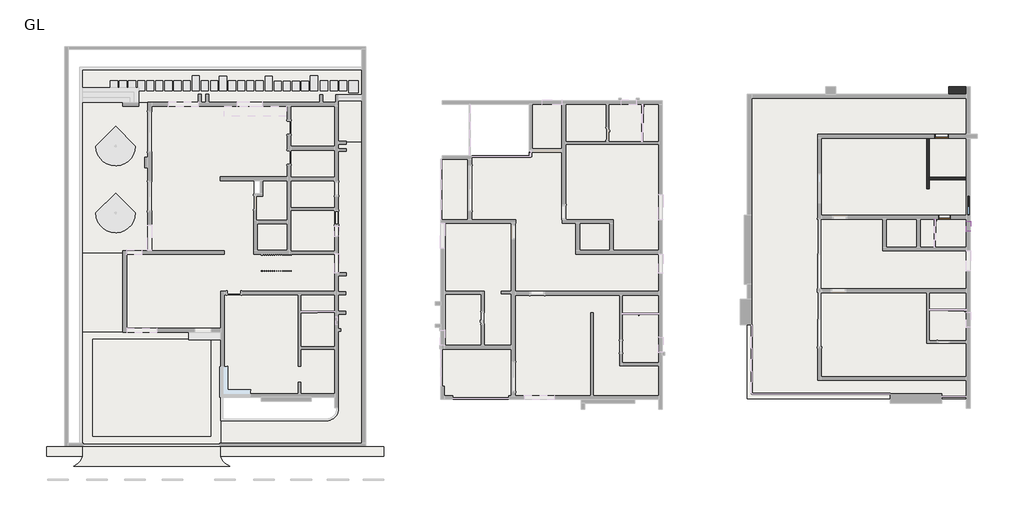
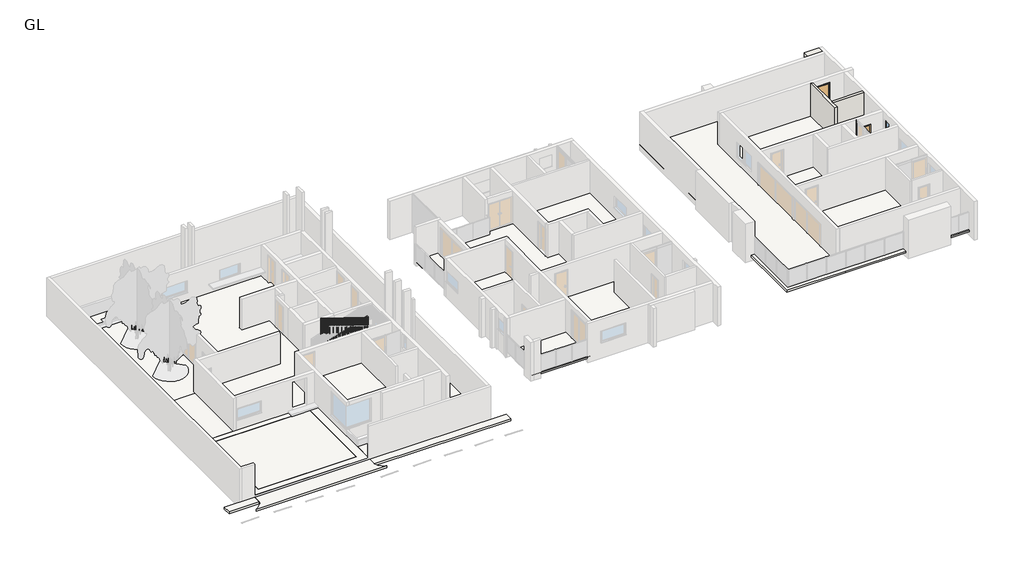
# One storey, part 5 of 6: 20 slabs, 3 walls, 2 doors, 2 members, 2 windows, 1 railing.
# Revit data of these elements (continued)
# Materials (continued)
#   "BALCONY": class "Generic", colour RGB 120 120 120, transparency 0, Cost = 0
#   "LIFT FLOOR": class "Generic", colour RGB 120 120 120, transparency 0, Cost = 0
#   "OPEN TERRACE": class "Generic", colour RGB 120 120 120, transparency 0, Cost = 0
#   "TOILET": class "Generic", colour RGB 120 120 120, transparency 0, Cost = 0
#   "MAIN FLOOR HALL": class "Generic", colour RGB 120 120 120, transparency 0, Cost = 0
#   "Brick, Common": class "Masonry", colour RGB 170 100 105, transparency 0, Description = "Common brick", Cost = 0
#   "Window Reveal": colour RGB 255 255 255, transparency 0
#   "Window Glass": colour RGB 0 0 255, transparency 0.75
#   "Window Frame": colour RGB 249 249 249, transparency 0, Keynote = "L10", Cost = 0
#   "Window Architrave": colour RGB 255 255 255, transparency 0
#   "Glass": class "Glass", colour RGB 0 128 192, transparency 0.9, Description = "Soda Lime Glass", Cost = 0
#   "Aluminium": class "Metal", colour RGB 247 247 247, transparency 0, Description = "Aluminium 6061", Cost = 0
